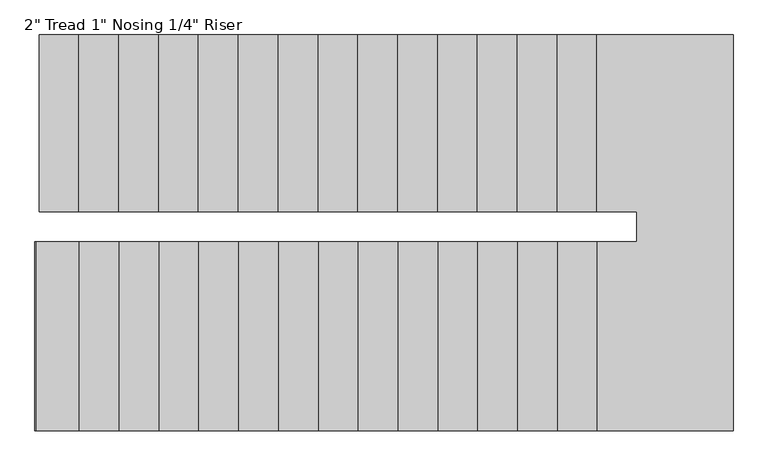
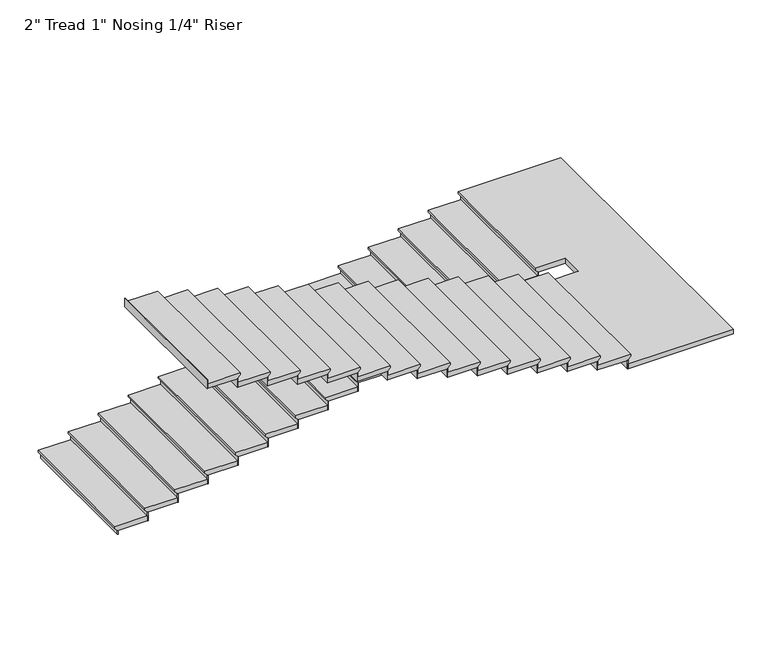
"""IFC4 building model written with IfcOpenShell, lengths in millimetres: stair flight geometry."""

from ifc_helpers import new_model, si_unit, origin, place, context, project, spatial, faceted_brep, source, transform, mapped, element, save


def stair_flight_175a6785(model_context):
    return source(origin(), model_context, "Body", "Brep", [
        faceted_brep([(-5254.0891351, 11154.2082924, 3120.39), (-5254.0891351, 11154.2082924, 3139.44), (-5254.0891351, 12506.0715905, 3139.44), (-5254.0891351, 12506.0715905, 3120.39), (-5228.6891351, 11154.2082924, 3094.99), (-5228.6891351, 12506.0715905, 3094.99), (-4923.8891351, 11154.2082924, 3139.44), (-4923.8891351, 12506.0715905, 3139.44), (-5228.6891351, 12506.0715905, 3088.64), (-4923.8891351, 12506.0715905, 3088.64), (-4923.8891351, 11154.2082924, 3088.64), (-5228.6891351, 11154.2082924, 3088.64)], [[[0, 1, 2, 3]], [[4, 0, 3, 5]], [[2, 1, 6, 7]], [[8, 9, 10, 11]], [[2, 7, 9, 8, 5, 3]], [[8, 11, 4, 5]], [[6, 1, 0, 4, 11, 10]], [[7, 6, 10, 9]]]),
        faceted_brep([(-5228.6891351, 11154.2082924, 3088.64), (-5228.6891351, 11154.2082924, 3048.0), (-5222.3391351, 11154.2082924, 3048.0), (-5222.3391351, 11154.2082924, 3088.64), (-5228.6891351, 12506.0715905, 3088.64), (-5222.3391351, 12506.0715905, 3088.64), (-5222.3391351, 12506.0715905, 3048.0), (-5228.6891351, 12506.0715905, 3048.0)], [[[0, 1, 2, 3]], [[4, 5, 6, 7]], [[1, 0, 4, 7]], [[2, 1, 7, 6]], [[3, 2, 6, 5]], [[0, 3, 5, 4]]]),
        faceted_brep([(-4923.8891351, 11154.2082924, 3180.08), (-4923.8891351, 11154.2082924, 3088.64), (-4917.5391351, 11154.2082924, 3088.64), (-4917.5391351, 11154.2082924, 3180.08), (-4923.8891351, 12506.0715905, 3180.08), (-4917.5391351, 12506.0715905, 3180.08), (-4917.5391351, 12506.0715905, 3088.64), (-4923.8891351, 12506.0715905, 3088.64)], [[[0, 1, 2, 3]], [[4, 5, 6, 7]], [[1, 0, 4, 7]], [[2, 1, 7, 6]], [[3, 2, 6, 5]], [[0, 3, 5, 4]]]),
        faceted_brep([(-4949.2891351, 12506.0715905, 3230.88), (-4949.2891351, 11154.2082924, 3230.88), (-4619.0891351, 11154.2082924, 3230.88), (-4619.0891351, 12506.0715905, 3230.88), (-4923.8891351, 12506.0715905, 3180.08), (-4619.0891351, 12506.0715905, 3180.08), (-4619.0891351, 11154.2082924, 3180.08), (-4923.8891351, 11154.2082924, 3180.08), (-4923.8891351, 12506.0715905, 3186.43), (-4949.2891351, 12506.0715905, 3211.83), (-4923.8891351, 11154.2082924, 3186.43), (-4949.2891351, 11154.2082924, 3211.83)], [[[0, 1, 2, 3]], [[4, 5, 6, 7]], [[0, 3, 5, 4, 8, 9]], [[4, 7, 10, 8]], [[2, 1, 11, 10, 7, 6]], [[3, 2, 6, 5]], [[11, 1, 0, 9]], [[10, 11, 9, 8]]]),
        faceted_brep([(-4619.0891351, 11154.2082924, 3271.52), (-4619.0891351, 11154.2082924, 3180.08), (-4612.7391351, 11154.2082924, 3180.08), (-4612.7391351, 11154.2082924, 3271.52), (-4619.0891351, 12506.0715905, 3271.52), (-4612.7391351, 12506.0715905, 3271.52), (-4612.7391351, 12506.0715905, 3180.08), (-4619.0891351, 12506.0715905, 3180.08)], [[[0, 1, 2, 3]], [[4, 5, 6, 7]], [[1, 0, 4, 7]], [[2, 1, 7, 6]], [[3, 2, 6, 5]], [[0, 3, 5, 4]]]),
        faceted_brep([(-4644.4891351, 12506.0715905, 3322.32), (-4644.4891351, 11154.2082924, 3322.32), (-4314.2891351, 11154.2082924, 3322.32), (-4314.2891351, 12506.0715905, 3322.32), (-4619.0891351, 12506.0715905, 3271.52), (-4314.2891351, 12506.0715905, 3271.52), (-4314.2891351, 11154.2082924, 3271.52), (-4619.0891351, 11154.2082924, 3271.52), (-4619.0891351, 12506.0715905, 3277.87), (-4644.4891351, 12506.0715905, 3303.27), (-4619.0891351, 11154.2082924, 3277.87), (-4644.4891351, 11154.2082924, 3303.27)], [[[0, 1, 2, 3]], [[4, 5, 6, 7]], [[0, 3, 5, 4, 8, 9]], [[4, 7, 10, 8]], [[2, 1, 11, 10, 7, 6]], [[3, 2, 6, 5]], [[11, 1, 0, 9]], [[10, 11, 9, 8]]]),
        faceted_brep([(-4314.2891351, 11154.2082924, 3362.96), (-4314.2891351, 11154.2082924, 3271.52), (-4307.9391351, 11154.2082924, 3271.52), (-4307.9391351, 11154.2082924, 3362.96), (-4314.2891351, 12506.0715905, 3362.96), (-4307.9391351, 12506.0715905, 3362.96), (-4307.9391351, 12506.0715905, 3271.52), (-4314.2891351, 12506.0715905, 3271.52)], [[[0, 1, 2, 3]], [[4, 5, 6, 7]], [[1, 0, 4, 7]], [[2, 1, 7, 6]], [[3, 2, 6, 5]], [[0, 3, 5, 4]]]),
        faceted_brep([(-4339.6891351, 12506.0715905, 3413.76), (-4339.6891351, 11154.2082924, 3413.76), (-4009.4891351, 11154.2082924, 3413.76), (-4009.4891351, 12506.0715905, 3413.76), (-4314.2891351, 12506.0715905, 3362.96), (-4009.4891351, 12506.0715905, 3362.96), (-4009.4891351, 11154.2082924, 3362.96), (-4314.2891351, 11154.2082924, 3362.96), (-4314.2891351, 12506.0715905, 3369.31), (-4339.6891351, 12506.0715905, 3394.71), (-4314.2891351, 11154.2082924, 3369.31), (-4339.6891351, 11154.2082924, 3394.71)], [[[0, 1, 2, 3]], [[4, 5, 6, 7]], [[0, 3, 5, 4, 8, 9]], [[4, 7, 10, 8]], [[2, 1, 11, 10, 7, 6]], [[3, 2, 6, 5]], [[11, 1, 0, 9]], [[10, 11, 9, 8]]]),
        faceted_brep([(-4009.4891351, 11154.2082924, 3454.4), (-4009.4891351, 11154.2082924, 3362.96), (-4003.1391351, 11154.2082924, 3362.96), (-4003.1391351, 11154.2082924, 3454.4), (-4009.4891351, 12506.0715905, 3454.4), (-4003.1391351, 12506.0715905, 3454.4), (-4003.1391351, 12506.0715905, 3362.96), (-4009.4891351, 12506.0715905, 3362.96)], [[[0, 1, 2, 3]], [[4, 5, 6, 7]], [[1, 0, 4, 7]], [[2, 1, 7, 6]], [[3, 2, 6, 5]], [[0, 3, 5, 4]]]),
        faceted_brep([(-4034.8891351, 12506.0715905, 3505.2), (-4034.8891351, 11154.2082924, 3505.2), (-3704.6891351, 11154.2082924, 3505.2), (-3704.6891351, 12506.0715905, 3505.2), (-4009.4891351, 12506.0715905, 3454.4), (-3704.6891351, 12506.0715905, 3454.4), (-3704.6891351, 11154.2082924, 3454.4), (-4009.4891351, 11154.2082924, 3454.4), (-4009.4891351, 12506.0715905, 3460.75), (-4034.8891351, 12506.0715905, 3486.15), (-4009.4891351, 11154.2082924, 3460.75), (-4034.8891351, 11154.2082924, 3486.15)], [[[0, 1, 2, 3]], [[4, 5, 6, 7]], [[0, 3, 5, 4, 8, 9]], [[4, 7, 10, 8]], [[2, 1, 11, 10, 7, 6]], [[3, 2, 6, 5]], [[11, 1, 0, 9]], [[10, 11, 9, 8]]]),
        faceted_brep([(-3704.6891351, 11154.2082924, 3545.84), (-3704.6891351, 11154.2082924, 3454.4), (-3698.3391351, 11154.2082924, 3454.4), (-3698.3391351, 11154.2082924, 3545.84), (-3704.6891351, 12506.0715905, 3545.84), (-3698.3391351, 12506.0715905, 3545.84), (-3698.3391351, 12506.0715905, 3454.4), (-3704.6891351, 12506.0715905, 3454.4)], [[[0, 1, 2, 3]], [[4, 5, 6, 7]], [[1, 0, 4, 7]], [[2, 1, 7, 6]], [[3, 2, 6, 5]], [[0, 3, 5, 4]]]),
        faceted_brep([(-3730.0891351, 12506.0715905, 3596.64), (-3730.0891351, 11154.2082924, 3596.64), (-3399.8891351, 11154.2082924, 3596.64), (-3399.8891351, 12506.0715905, 3596.64), (-3704.6891351, 12506.0715905, 3545.84), (-3399.8891351, 12506.0715905, 3545.84), (-3399.8891351, 11154.2082924, 3545.84), (-3704.6891351, 11154.2082924, 3545.84), (-3704.6891351, 12506.0715905, 3552.19), (-3730.0891351, 12506.0715905, 3577.59), (-3704.6891351, 11154.2082924, 3552.19), (-3730.0891351, 11154.2082924, 3577.59)], [[[0, 1, 2, 3]], [[4, 5, 6, 7]], [[0, 3, 5, 4, 8, 9]], [[4, 7, 10, 8]], [[2, 1, 11, 10, 7, 6]], [[3, 2, 6, 5]], [[11, 1, 0, 9]], [[10, 11, 9, 8]]]),
        faceted_brep([(-3399.8891351, 11154.2082924, 3637.28), (-3399.8891351, 11154.2082924, 3545.84), (-3393.5391351, 11154.2082924, 3545.84), (-3393.5391351, 11154.2082924, 3637.28), (-3399.8891351, 12506.0715905, 3637.28), (-3393.5391351, 12506.0715905, 3637.28), (-3393.5391351, 12506.0715905, 3545.84), (-3399.8891351, 12506.0715905, 3545.84)], [[[0, 1, 2, 3]], [[4, 5, 6, 7]], [[1, 0, 4, 7]], [[2, 1, 7, 6]], [[3, 2, 6, 5]], [[0, 3, 5, 4]]]),
        faceted_brep([(-3425.2891351, 12506.0715905, 3688.08), (-3425.2891351, 11154.2082924, 3688.08), (-3095.0891351, 11154.2082924, 3688.08), (-3095.0891351, 12506.0715905, 3688.08), (-3399.8891351, 12506.0715905, 3637.28), (-3095.0891351, 12506.0715905, 3637.28), (-3095.0891351, 11154.2082924, 3637.28), (-3399.8891351, 11154.2082924, 3637.28), (-3399.8891351, 12506.0715905, 3643.63), (-3425.2891351, 12506.0715905, 3669.03), (-3399.8891351, 11154.2082924, 3643.63), (-3425.2891351, 11154.2082924, 3669.03)], [[[0, 1, 2, 3]], [[4, 5, 6, 7]], [[0, 3, 5, 4, 8, 9]], [[4, 7, 10, 8]], [[2, 1, 11, 10, 7, 6]], [[3, 2, 6, 5]], [[11, 1, 0, 9]], [[10, 11, 9, 8]]]),
        faceted_brep([(-3095.0891351, 11154.2082924, 3728.72), (-3095.0891351, 11154.2082924, 3637.28), (-3088.7391351, 11154.2082924, 3637.28), (-3088.7391351, 11154.2082924, 3728.72), (-3095.0891351, 12506.0715905, 3728.72), (-3088.7391351, 12506.0715905, 3728.72), (-3088.7391351, 12506.0715905, 3637.28), (-3095.0891351, 12506.0715905, 3637.28)], [[[0, 1, 2, 3]], [[4, 5, 6, 7]], [[1, 0, 4, 7]], [[2, 1, 7, 6]], [[3, 2, 6, 5]], [[0, 3, 5, 4]]]),
        faceted_brep([(-3120.4891351, 12506.0715905, 3779.52), (-3120.4891351, 11154.2082924, 3779.52), (-2790.2891351, 11154.2082924, 3779.52), (-2790.2891351, 12506.0715905, 3779.52), (-3095.0891351, 12506.0715905, 3728.72), (-2790.2891351, 12506.0715905, 3728.72), (-2790.2891351, 11154.2082924, 3728.72), (-3095.0891351, 11154.2082924, 3728.72), (-3095.0891351, 12506.0715905, 3735.07), (-3120.4891351, 12506.0715905, 3760.47), (-3095.0891351, 11154.2082924, 3735.07), (-3120.4891351, 11154.2082924, 3760.47)], [[[0, 1, 2, 3]], [[4, 5, 6, 7]], [[0, 3, 5, 4, 8, 9]], [[4, 7, 10, 8]], [[2, 1, 11, 10, 7, 6]], [[3, 2, 6, 5]], [[11, 1, 0, 9]], [[10, 11, 9, 8]]]),
        faceted_brep([(-2790.2891351, 11154.2082924, 3820.16), (-2790.2891351, 11154.2082924, 3728.72), (-2783.9391351, 11154.2082924, 3728.72), (-2783.9391351, 11154.2082924, 3820.16), (-2790.2891351, 12506.0715905, 3820.16), (-2783.9391351, 12506.0715905, 3820.16), (-2783.9391351, 12506.0715905, 3728.72), (-2790.2891351, 12506.0715905, 3728.72)], [[[0, 1, 2, 3]], [[4, 5, 6, 7]], [[1, 0, 4, 7]], [[2, 1, 7, 6]], [[3, 2, 6, 5]], [[0, 3, 5, 4]]]),
        faceted_brep([(-2815.6891351, 12506.0715905, 3870.96), (-2815.6891351, 11154.2082924, 3870.96), (-2485.4891351, 11154.2082924, 3870.96), (-2485.4891351, 12506.0715905, 3870.96), (-2790.2891351, 12506.0715905, 3820.16), (-2485.4891351, 12506.0715905, 3820.16), (-2485.4891351, 11154.2082924, 3820.16), (-2790.2891351, 11154.2082924, 3820.16), (-2790.2891351, 12506.0715905, 3826.51), (-2815.6891351, 12506.0715905, 3851.91), (-2790.2891351, 11154.2082924, 3826.51), (-2815.6891351, 11154.2082924, 3851.91)], [[[0, 1, 2, 3]], [[4, 5, 6, 7]], [[0, 3, 5, 4, 8, 9]], [[4, 7, 10, 8]], [[2, 1, 11, 10, 7, 6]], [[3, 2, 6, 5]], [[11, 1, 0, 9]], [[10, 11, 9, 8]]]),
        faceted_brep([(-2485.4891351, 11154.2082924, 3911.6), (-2485.4891351, 11154.2082924, 3820.16), (-2479.1391351, 11154.2082924, 3820.16), (-2479.1391351, 11154.2082924, 3911.6), (-2485.4891351, 12506.0715905, 3911.6), (-2479.1391351, 12506.0715905, 3911.6), (-2479.1391351, 12506.0715905, 3820.16), (-2485.4891351, 12506.0715905, 3820.16)], [[[0, 1, 2, 3]], [[4, 5, 6, 7]], [[1, 0, 4, 7]], [[2, 1, 7, 6]], [[3, 2, 6, 5]], [[0, 3, 5, 4]]]),
        faceted_brep([(-2510.8891351, 12506.0715905, 3962.4), (-2510.8891351, 11154.2082924, 3962.4), (-2180.6891351, 11154.2082924, 3962.4), (-2180.6891351, 12506.0715905, 3962.4), (-2485.4891351, 12506.0715905, 3911.6), (-2180.6891351, 12506.0715905, 3911.6), (-2180.6891351, 11154.2082924, 3911.6), (-2485.4891351, 11154.2082924, 3911.6), (-2485.4891351, 12506.0715905, 3917.95), (-2510.8891351, 12506.0715905, 3943.35), (-2485.4891351, 11154.2082924, 3917.95), (-2510.8891351, 11154.2082924, 3943.35)], [[[0, 1, 2, 3]], [[4, 5, 6, 7]], [[0, 3, 5, 4, 8, 9]], [[4, 7, 10, 8]], [[2, 1, 11, 10, 7, 6]], [[3, 2, 6, 5]], [[11, 1, 0, 9]], [[10, 11, 9, 8]]]),
        faceted_brep([(-2180.6891351, 11154.2082924, 4003.04), (-2180.6891351, 11154.2082924, 3911.6), (-2174.3391351, 11154.2082924, 3911.6), (-2174.3391351, 11154.2082924, 4003.04), (-2180.6891351, 12506.0715905, 4003.04), (-2174.3391351, 12506.0715905, 4003.04), (-2174.3391351, 12506.0715905, 3911.6), (-2180.6891351, 12506.0715905, 3911.6)], [[[0, 1, 2, 3]], [[4, 5, 6, 7]], [[1, 0, 4, 7]], [[2, 1, 7, 6]], [[3, 2, 6, 5]], [[0, 3, 5, 4]]]),
        faceted_brep([(-2206.0891351, 12506.0715905, 4053.84), (-2206.0891351, 11154.2082924, 4053.84), (-1875.8891351, 11154.2082924, 4053.84), (-1875.8891351, 12506.0715905, 4053.84), (-2180.6891351, 12506.0715905, 4003.04), (-1875.8891351, 12506.0715905, 4003.04), (-1875.8891351, 11154.2082924, 4003.04), (-2180.6891351, 11154.2082924, 4003.04), (-2180.6891351, 12506.0715905, 4009.39), (-2206.0891351, 12506.0715905, 4034.79), (-2180.6891351, 11154.2082924, 4009.39), (-2206.0891351, 11154.2082924, 4034.79)], [[[0, 1, 2, 3]], [[4, 5, 6, 7]], [[0, 3, 5, 4, 8, 9]], [[4, 7, 10, 8]], [[2, 1, 11, 10, 7, 6]], [[3, 2, 6, 5]], [[11, 1, 0, 9]], [[10, 11, 9, 8]]]),
        faceted_brep([(-1875.8891351, 11154.2082924, 4094.48), (-1875.8891351, 11154.2082924, 4003.04), (-1869.5391351, 11154.2082924, 4003.04), (-1869.5391351, 11154.2082924, 4094.48), (-1875.8891351, 12506.0715905, 4094.48), (-1869.5391351, 12506.0715905, 4094.48), (-1869.5391351, 12506.0715905, 4003.04), (-1875.8891351, 12506.0715905, 4003.04)], [[[0, 1, 2, 3]], [[4, 5, 6, 7]], [[1, 0, 4, 7]], [[2, 1, 7, 6]], [[3, 2, 6, 5]], [[0, 3, 5, 4]]]),
        faceted_brep([(-1901.2891351, 12506.0715905, 4145.28), (-1901.2891351, 11154.2082924, 4145.28), (-1571.0891351, 11154.2082924, 4145.28), (-1571.0891351, 12506.0715905, 4145.28), (-1875.8891351, 12506.0715905, 4094.48), (-1571.0891351, 12506.0715905, 4094.48), (-1571.0891351, 11154.2082924, 4094.48), (-1875.8891351, 11154.2082924, 4094.48), (-1875.8891351, 12506.0715905, 4100.83), (-1901.2891351, 12506.0715905, 4126.23), (-1875.8891351, 11154.2082924, 4100.83), (-1901.2891351, 11154.2082924, 4126.23)], [[[0, 1, 2, 3]], [[4, 5, 6, 7]], [[0, 3, 5, 4, 8, 9]], [[4, 7, 10, 8]], [[2, 1, 11, 10, 7, 6]], [[3, 2, 6, 5]], [[11, 1, 0, 9]], [[10, 11, 9, 8]]]),
        faceted_brep([(-1571.0891351, 11154.2082924, 4185.92), (-1571.0891351, 11154.2082924, 4094.48), (-1564.7391351, 11154.2082924, 4094.48), (-1564.7391351, 11154.2082924, 4185.92), (-1571.0891351, 12506.0715905, 4185.92), (-1564.7391351, 12506.0715905, 4185.92), (-1564.7391351, 12506.0715905, 4094.48), (-1571.0891351, 12506.0715905, 4094.48)], [[[0, 1, 2, 3]], [[4, 5, 6, 7]], [[1, 0, 4, 7]], [[2, 1, 7, 6]], [[3, 2, 6, 5]], [[0, 3, 5, 4]]]),
        faceted_brep([(-1596.4891351, 12506.0715905, 4236.72), (-1596.4891351, 11154.2082924, 4236.72), (-1266.2891351, 11154.2082924, 4236.72), (-1266.2891351, 12506.0715905, 4236.72), (-1571.0891351, 12506.0715905, 4185.92), (-1266.2891351, 12506.0715905, 4185.92), (-1266.2891351, 11154.2082924, 4185.92), (-1571.0891351, 11154.2082924, 4185.92), (-1571.0891351, 12506.0715905, 4192.27), (-1596.4891351, 12506.0715905, 4217.67), (-1571.0891351, 11154.2082924, 4192.27), (-1596.4891351, 11154.2082924, 4217.67)], [[[0, 1, 2, 3]], [[4, 5, 6, 7]], [[0, 3, 5, 4, 8, 9]], [[4, 7, 10, 8]], [[2, 1, 11, 10, 7, 6]], [[3, 2, 6, 5]], [[11, 1, 0, 9]], [[10, 11, 9, 8]]]),
        faceted_brep([(-1266.2891351, 11154.2082924, 4277.36), (-1266.2891351, 11154.2082924, 4185.92), (-1259.9391351, 11154.2082924, 4185.92), (-1259.9391351, 11154.2082924, 4277.36), (-1266.2891351, 12506.0715905, 4277.36), (-1259.9391351, 12506.0715905, 4277.36), (-1259.9391351, 12506.0715905, 4185.92), (-1266.2891351, 12506.0715905, 4185.92)], [[[0, 1, 2, 3]], [[4, 5, 6, 7]], [[1, 0, 4, 7]], [[2, 1, 7, 6]], [[3, 2, 6, 5]], [[0, 3, 5, 4]]]),
        faceted_brep([(-1291.6891351, 12506.0715905, 4328.16), (-1291.6891351, 11154.2082924, 4328.16), (-961.4891351, 11154.2082924, 4328.16), (-961.4891351, 12506.0715905, 4328.16), (-1266.2891351, 12506.0715905, 4277.36), (-961.4891351, 12506.0715905, 4277.36), (-961.4891351, 11154.2082924, 4277.36), (-1266.2891351, 11154.2082924, 4277.36), (-1266.2891351, 12506.0715905, 4283.71), (-1291.6891351, 12506.0715905, 4309.11), (-1266.2891351, 11154.2082924, 4283.71), (-1291.6891351, 11154.2082924, 4309.11)], [[[0, 1, 2, 3]], [[4, 5, 6, 7]], [[0, 3, 5, 4, 8, 9]], [[4, 7, 10, 8]], [[2, 1, 11, 10, 7, 6]], [[3, 2, 6, 5]], [[11, 1, 0, 9]], [[10, 11, 9, 8]]]),
        faceted_brep([(-961.4891351, 11154.2082924, 4368.8), (-961.4891351, 11154.2082924, 4277.36), (-955.1391351, 11154.2082924, 4277.36), (-955.1391351, 11154.2082924, 4368.8), (-961.4891351, 12506.0715905, 4368.8), (-955.1391351, 12506.0715905, 4368.8), (-955.1391351, 12506.0715905, 4277.36), (-961.4891351, 12506.0715905, 4277.36)], [[[0, 1, 2, 3]], [[4, 5, 6, 7]], [[1, 0, 4, 7]], [[2, 1, 7, 6]], [[3, 2, 6, 5]], [[0, 3, 5, 4]]]),
        faceted_brep([(-1012.2891351, 9478.4949943, 4419.6), (54.5108649, 9478.4949943, 4419.6), (54.5108649, 12506.0715905, 4419.6), (-986.8891351, 12506.0715905, 4419.6), (-986.8891351, 11154.2082924, 4419.6), (-682.0891351, 11154.2082924, 4419.6), (-682.0891351, 10925.6082924, 4419.6), (-1012.2891351, 10925.6082924, 4419.6), (54.5108649, 9478.4949943, 4368.8), (-1012.2891351, 9478.4949943, 4368.8), (-1012.2891351, 10925.6082924, 4368.8), (-682.0891351, 10925.6082924, 4368.8), (-682.0891351, 11154.2082924, 4368.8), (-961.4891351, 11154.2082924, 4368.8), (-961.4891351, 12506.0715905, 4368.8), (54.5108649, 12506.0715905, 4368.8), (-961.4891351, 12506.0715905, 4375.15), (-986.8891351, 12506.0715905, 4400.55), (-961.4891351, 11154.2082924, 4375.15), (-986.8891351, 11154.2082924, 4400.55)], [[[0, 1, 2, 3, 4, 5, 6, 7]], [[8, 9, 10, 11, 12, 13, 14, 15]], [[1, 0, 9, 8]], [[2, 1, 8, 15]], [[3, 2, 15, 14, 16, 17]], [[14, 13, 18, 16]], [[5, 4, 19, 18, 13, 12]], [[6, 5, 12, 11]], [[7, 6, 11, 10]], [[0, 7, 10, 9]], [[19, 4, 3, 17]], [[18, 19, 17, 16]]]),
        faceted_brep([(-1012.2891351, 10925.6082924, 4460.24), (-1012.2891351, 10925.6082924, 4368.8), (-1018.6391351, 10925.6082924, 4368.8), (-1018.6391351, 10925.6082924, 4460.24), (-1012.2891351, 9478.4949943, 4460.24), (-1018.6391351, 9478.4949943, 4460.24), (-1018.6391351, 9478.4949943, 4368.8), (-1012.2891351, 9478.4949943, 4368.8)], [[[0, 1, 2, 3]], [[4, 5, 6, 7]], [[1, 0, 4, 7]], [[2, 1, 7, 6]], [[3, 2, 6, 5]], [[0, 3, 5, 4]]]),
        faceted_brep([(-986.8891351, 9478.4949943, 4511.04), (-986.8891351, 10925.6082924, 4511.04), (-1317.0891351, 10925.6082924, 4511.04), (-1317.0891351, 9478.4949943, 4511.04), (-1012.2891351, 9478.4949943, 4460.24), (-1317.0891351, 9478.4949943, 4460.24), (-1317.0891351, 10925.6082924, 4460.24), (-1012.2891351, 10925.6082924, 4460.24), (-1012.2891351, 9478.4949943, 4466.59), (-986.8891351, 9478.4949943, 4491.99), (-1012.2891351, 10925.6082924, 4466.59), (-986.8891351, 10925.6082924, 4491.99)], [[[0, 1, 2, 3]], [[4, 5, 6, 7]], [[0, 3, 5, 4, 8, 9]], [[4, 7, 10, 8]], [[2, 1, 11, 10, 7, 6]], [[3, 2, 6, 5]], [[11, 1, 0, 9]], [[10, 11, 9, 8]]]),
        faceted_brep([(-1317.0891351, 10925.6082924, 4551.68), (-1317.0891351, 10925.6082924, 4460.24), (-1323.4391351, 10925.6082924, 4460.24), (-1323.4391351, 10925.6082924, 4551.68), (-1317.0891351, 9478.4949943, 4551.68), (-1323.4391351, 9478.4949943, 4551.68), (-1323.4391351, 9478.4949943, 4460.24), (-1317.0891351, 9478.4949943, 4460.24)], [[[0, 1, 2, 3]], [[4, 5, 6, 7]], [[1, 0, 4, 7]], [[2, 1, 7, 6]], [[3, 2, 6, 5]], [[0, 3, 5, 4]]]),
        faceted_brep([(-1291.6891351, 9478.4949943, 4602.48), (-1291.6891351, 10925.6082924, 4602.48), (-1621.8891351, 10925.6082924, 4602.48), (-1621.8891351, 9478.4949943, 4602.48), (-1317.0891351, 9478.4949943, 4551.68), (-1621.8891351, 9478.4949943, 4551.68), (-1621.8891351, 10925.6082924, 4551.68), (-1317.0891351, 10925.6082924, 4551.68), (-1317.0891351, 9478.4949943, 4558.03), (-1291.6891351, 9478.4949943, 4583.43), (-1317.0891351, 10925.6082924, 4558.03), (-1291.6891351, 10925.6082924, 4583.43)], [[[0, 1, 2, 3]], [[4, 5, 6, 7]], [[0, 3, 5, 4, 8, 9]], [[4, 7, 10, 8]], [[2, 1, 11, 10, 7, 6]], [[3, 2, 6, 5]], [[11, 1, 0, 9]], [[10, 11, 9, 8]]]),
        faceted_brep([(-1621.8891351, 10925.6082924, 4643.12), (-1621.8891351, 10925.6082924, 4551.68), (-1628.2391351, 10925.6082924, 4551.68), (-1628.2391351, 10925.6082924, 4643.12), (-1621.8891351, 9478.4949943, 4643.12), (-1628.2391351, 9478.4949943, 4643.12), (-1628.2391351, 9478.4949943, 4551.68), (-1621.8891351, 9478.4949943, 4551.68)], [[[0, 1, 2, 3]], [[4, 5, 6, 7]], [[1, 0, 4, 7]], [[2, 1, 7, 6]], [[3, 2, 6, 5]], [[0, 3, 5, 4]]]),
        faceted_brep([(-1596.4891351, 9478.4949943, 4693.92), (-1596.4891351, 10925.6082924, 4693.92), (-1926.6891351, 10925.6082924, 4693.92), (-1926.6891351, 9478.4949943, 4693.92), (-1621.8891351, 9478.4949943, 4643.12), (-1926.6891351, 9478.4949943, 4643.12), (-1926.6891351, 10925.6082924, 4643.12), (-1621.8891351, 10925.6082924, 4643.12), (-1621.8891351, 9478.4949943, 4649.47), (-1596.4891351, 9478.4949943, 4674.87), (-1621.8891351, 10925.6082924, 4649.47), (-1596.4891351, 10925.6082924, 4674.87)], [[[0, 1, 2, 3]], [[4, 5, 6, 7]], [[0, 3, 5, 4, 8, 9]], [[4, 7, 10, 8]], [[2, 1, 11, 10, 7, 6]], [[3, 2, 6, 5]], [[11, 1, 0, 9]], [[10, 11, 9, 8]]]),
        faceted_brep([(-1926.6891351, 10925.6082924, 4734.56), (-1926.6891351, 10925.6082924, 4643.12), (-1933.0391351, 10925.6082924, 4643.12), (-1933.0391351, 10925.6082924, 4734.56), (-1926.6891351, 9478.4949943, 4734.56), (-1933.0391351, 9478.4949943, 4734.56), (-1933.0391351, 9478.4949943, 4643.12), (-1926.6891351, 9478.4949943, 4643.12)], [[[0, 1, 2, 3]], [[4, 5, 6, 7]], [[1, 0, 4, 7]], [[2, 1, 7, 6]], [[3, 2, 6, 5]], [[0, 3, 5, 4]]]),
        faceted_brep([(-1901.2891351, 9478.4949943, 4785.36), (-1901.2891351, 10925.6082924, 4785.36), (-2231.4891351, 10925.6082924, 4785.36), (-2231.4891351, 9478.4949943, 4785.36), (-1926.6891351, 9478.4949943, 4734.56), (-2231.4891351, 9478.4949943, 4734.56), (-2231.4891351, 10925.6082924, 4734.56), (-1926.6891351, 10925.6082924, 4734.56), (-1926.6891351, 9478.4949943, 4740.91), (-1901.2891351, 9478.4949943, 4766.31), (-1926.6891351, 10925.6082924, 4740.91), (-1901.2891351, 10925.6082924, 4766.31)], [[[0, 1, 2, 3]], [[4, 5, 6, 7]], [[0, 3, 5, 4, 8, 9]], [[4, 7, 10, 8]], [[2, 1, 11, 10, 7, 6]], [[3, 2, 6, 5]], [[11, 1, 0, 9]], [[10, 11, 9, 8]]]),
        faceted_brep([(-2231.4891351, 10925.6082924, 4826.0), (-2231.4891351, 10925.6082924, 4734.56), (-2237.8391351, 10925.6082924, 4734.56), (-2237.8391351, 10925.6082924, 4826.0), (-2231.4891351, 9478.4949943, 4826.0), (-2237.8391351, 9478.4949943, 4826.0), (-2237.8391351, 9478.4949943, 4734.56), (-2231.4891351, 9478.4949943, 4734.56)], [[[0, 1, 2, 3]], [[4, 5, 6, 7]], [[1, 0, 4, 7]], [[2, 1, 7, 6]], [[3, 2, 6, 5]], [[0, 3, 5, 4]]]),
        faceted_brep([(-2206.0891351, 9478.4949943, 4876.8), (-2206.0891351, 10925.6082924, 4876.8), (-2536.2891351, 10925.6082924, 4876.8), (-2536.2891351, 9478.4949943, 4876.8), (-2231.4891351, 9478.4949943, 4826.0), (-2536.2891351, 9478.4949943, 4826.0), (-2536.2891351, 10925.6082924, 4826.0), (-2231.4891351, 10925.6082924, 4826.0), (-2231.4891351, 9478.4949943, 4832.35), (-2206.0891351, 9478.4949943, 4857.75), (-2231.4891351, 10925.6082924, 4832.35), (-2206.0891351, 10925.6082924, 4857.75)], [[[0, 1, 2, 3]], [[4, 5, 6, 7]], [[0, 3, 5, 4, 8, 9]], [[4, 7, 10, 8]], [[2, 1, 11, 10, 7, 6]], [[3, 2, 6, 5]], [[11, 1, 0, 9]], [[10, 11, 9, 8]]]),
        faceted_brep([(-2536.2891351, 10925.6082924, 4917.44), (-2536.2891351, 10925.6082924, 4826.0), (-2542.6391351, 10925.6082924, 4826.0), (-2542.6391351, 10925.6082924, 4917.44), (-2536.2891351, 9478.4949943, 4917.44), (-2542.6391351, 9478.4949943, 4917.44), (-2542.6391351, 9478.4949943, 4826.0), (-2536.2891351, 9478.4949943, 4826.0)], [[[0, 1, 2, 3]], [[4, 5, 6, 7]], [[1, 0, 4, 7]], [[2, 1, 7, 6]], [[3, 2, 6, 5]], [[0, 3, 5, 4]]]),
        faceted_brep([(-2510.8891351, 9478.4949943, 4968.24), (-2510.8891351, 10925.6082924, 4968.24), (-2841.0891351, 10925.6082924, 4968.24), (-2841.0891351, 9478.4949943, 4968.24), (-2536.2891351, 9478.4949943, 4917.44), (-2841.0891351, 9478.4949943, 4917.44), (-2841.0891351, 10925.6082924, 4917.44), (-2536.2891351, 10925.6082924, 4917.44), (-2536.2891351, 9478.4949943, 4923.79), (-2510.8891351, 9478.4949943, 4949.19), (-2536.2891351, 10925.6082924, 4923.79), (-2510.8891351, 10925.6082924, 4949.19)], [[[0, 1, 2, 3]], [[4, 5, 6, 7]], [[0, 3, 5, 4, 8, 9]], [[4, 7, 10, 8]], [[2, 1, 11, 10, 7, 6]], [[3, 2, 6, 5]], [[11, 1, 0, 9]], [[10, 11, 9, 8]]]),
        faceted_brep([(-2841.0891351, 10925.6082924, 5008.88), (-2841.0891351, 10925.6082924, 4917.44), (-2847.4391351, 10925.6082924, 4917.44), (-2847.4391351, 10925.6082924, 5008.88), (-2841.0891351, 9478.4949943, 5008.88), (-2847.4391351, 9478.4949943, 5008.88), (-2847.4391351, 9478.4949943, 4917.44), (-2841.0891351, 9478.4949943, 4917.44)], [[[0, 1, 2, 3]], [[4, 5, 6, 7]], [[1, 0, 4, 7]], [[2, 1, 7, 6]], [[3, 2, 6, 5]], [[0, 3, 5, 4]]]),
        faceted_brep([(-2815.6891351, 9478.4949943, 5059.68), (-2815.6891351, 10925.6082924, 5059.68), (-3145.8891351, 10925.6082924, 5059.68), (-3145.8891351, 9478.4949943, 5059.68), (-2841.0891351, 9478.4949943, 5008.88), (-3145.8891351, 9478.4949943, 5008.88), (-3145.8891351, 10925.6082924, 5008.88), (-2841.0891351, 10925.6082924, 5008.88), (-2841.0891351, 9478.4949943, 5015.23), (-2815.6891351, 9478.4949943, 5040.63), (-2841.0891351, 10925.6082924, 5015.23), (-2815.6891351, 10925.6082924, 5040.63)], [[[0, 1, 2, 3]], [[4, 5, 6, 7]], [[0, 3, 5, 4, 8, 9]], [[4, 7, 10, 8]], [[2, 1, 11, 10, 7, 6]], [[3, 2, 6, 5]], [[11, 1, 0, 9]], [[10, 11, 9, 8]]]),
        faceted_brep([(-3145.8891351, 10925.6082924, 5100.32), (-3145.8891351, 10925.6082924, 5008.88), (-3152.2391351, 10925.6082924, 5008.88), (-3152.2391351, 10925.6082924, 5100.32), (-3145.8891351, 9478.4949943, 5100.32), (-3152.2391351, 9478.4949943, 5100.32), (-3152.2391351, 9478.4949943, 5008.88), (-3145.8891351, 9478.4949943, 5008.88)], [[[0, 1, 2, 3]], [[4, 5, 6, 7]], [[1, 0, 4, 7]], [[2, 1, 7, 6]], [[3, 2, 6, 5]], [[0, 3, 5, 4]]]),
        faceted_brep([(-3120.4891351, 9478.4949943, 5151.12), (-3120.4891351, 10925.6082924, 5151.12), (-3450.6891351, 10925.6082924, 5151.12), (-3450.6891351, 9478.4949943, 5151.12), (-3145.8891351, 9478.4949943, 5100.32), (-3450.6891351, 9478.4949943, 5100.32), (-3450.6891351, 10925.6082924, 5100.32), (-3145.8891351, 10925.6082924, 5100.32), (-3145.8891351, 9478.4949943, 5106.67), (-3120.4891351, 9478.4949943, 5132.07), (-3145.8891351, 10925.6082924, 5106.67), (-3120.4891351, 10925.6082924, 5132.07)], [[[0, 1, 2, 3]], [[4, 5, 6, 7]], [[0, 3, 5, 4, 8, 9]], [[4, 7, 10, 8]], [[2, 1, 11, 10, 7, 6]], [[3, 2, 6, 5]], [[11, 1, 0, 9]], [[10, 11, 9, 8]]]),
        faceted_brep([(-3450.6891351, 10925.6082924, 5191.76), (-3450.6891351, 10925.6082924, 5100.32), (-3457.0391351, 10925.6082924, 5100.32), (-3457.0391351, 10925.6082924, 5191.76), (-3450.6891351, 9478.4949943, 5191.76), (-3457.0391351, 9478.4949943, 5191.76), (-3457.0391351, 9478.4949943, 5100.32), (-3450.6891351, 9478.4949943, 5100.32)], [[[0, 1, 2, 3]], [[4, 5, 6, 7]], [[1, 0, 4, 7]], [[2, 1, 7, 6]], [[3, 2, 6, 5]], [[0, 3, 5, 4]]]),
        faceted_brep([(-3425.2891351, 9478.4949943, 5242.56), (-3425.2891351, 10925.6082924, 5242.56), (-3755.4891351, 10925.6082924, 5242.56), (-3755.4891351, 9478.4949943, 5242.56), (-3450.6891351, 9478.4949943, 5191.76), (-3755.4891351, 9478.4949943, 5191.76), (-3755.4891351, 10925.6082924, 5191.76), (-3450.6891351, 10925.6082924, 5191.76), (-3450.6891351, 9478.4949943, 5198.11), (-3425.2891351, 9478.4949943, 5223.51), (-3450.6891351, 10925.6082924, 5198.11), (-3425.2891351, 10925.6082924, 5223.51)], [[[0, 1, 2, 3]], [[4, 5, 6, 7]], [[0, 3, 5, 4, 8, 9]], [[4, 7, 10, 8]], [[2, 1, 11, 10, 7, 6]], [[3, 2, 6, 5]], [[11, 1, 0, 9]], [[10, 11, 9, 8]]]),
        faceted_brep([(-3755.4891351, 10925.6082924, 5283.2), (-3755.4891351, 10925.6082924, 5191.76), (-3761.8391351, 10925.6082924, 5191.76), (-3761.8391351, 10925.6082924, 5283.2), (-3755.4891351, 9478.4949943, 5283.2), (-3761.8391351, 9478.4949943, 5283.2), (-3761.8391351, 9478.4949943, 5191.76), (-3755.4891351, 9478.4949943, 5191.76)], [[[0, 1, 2, 3]], [[4, 5, 6, 7]], [[1, 0, 4, 7]], [[2, 1, 7, 6]], [[3, 2, 6, 5]], [[0, 3, 5, 4]]]),
        faceted_brep([(-3730.0891351, 9478.4949943, 5334.0), (-3730.0891351, 10925.6082924, 5334.0), (-4060.2891351, 10925.6082924, 5334.0), (-4060.2891351, 9478.4949943, 5334.0), (-3755.4891351, 9478.4949943, 5283.2), (-4060.2891351, 9478.4949943, 5283.2), (-4060.2891351, 10925.6082924, 5283.2), (-3755.4891351, 10925.6082924, 5283.2), (-3755.4891351, 9478.4949943, 5289.55), (-3730.0891351, 9478.4949943, 5314.95), (-3755.4891351, 10925.6082924, 5289.55), (-3730.0891351, 10925.6082924, 5314.95)], [[[0, 1, 2, 3]], [[4, 5, 6, 7]], [[0, 3, 5, 4, 8, 9]], [[4, 7, 10, 8]], [[2, 1, 11, 10, 7, 6]], [[3, 2, 6, 5]], [[11, 1, 0, 9]], [[10, 11, 9, 8]]]),
        faceted_brep([(-4060.2891351, 10925.6082924, 5374.64), (-4060.2891351, 10925.6082924, 5283.2), (-4066.6391351, 10925.6082924, 5283.2), (-4066.6391351, 10925.6082924, 5374.64), (-4060.2891351, 9478.4949943, 5374.64), (-4066.6391351, 9478.4949943, 5374.64), (-4066.6391351, 9478.4949943, 5283.2), (-4060.2891351, 9478.4949943, 5283.2)], [[[0, 1, 2, 3]], [[4, 5, 6, 7]], [[1, 0, 4, 7]], [[2, 1, 7, 6]], [[3, 2, 6, 5]], [[0, 3, 5, 4]]]),
        faceted_brep([(-4034.8891351, 9478.4949943, 5425.44), (-4034.8891351, 10925.6082924, 5425.44), (-4365.0891351, 10925.6082924, 5425.44), (-4365.0891351, 9478.4949943, 5425.44), (-4060.2891351, 9478.4949943, 5374.64), (-4365.0891351, 9478.4949943, 5374.64), (-4365.0891351, 10925.6082924, 5374.64), (-4060.2891351, 10925.6082924, 5374.64), (-4060.2891351, 9478.4949943, 5380.99), (-4034.8891351, 9478.4949943, 5406.39), (-4060.2891351, 10925.6082924, 5380.99), (-4034.8891351, 10925.6082924, 5406.39)], [[[0, 1, 2, 3]], [[4, 5, 6, 7]], [[0, 3, 5, 4, 8, 9]], [[4, 7, 10, 8]], [[2, 1, 11, 10, 7, 6]], [[3, 2, 6, 5]], [[11, 1, 0, 9]], [[10, 11, 9, 8]]]),
        faceted_brep([(-4365.0891351, 10925.6082924, 5466.08), (-4365.0891351, 10925.6082924, 5374.64), (-4371.4391351, 10925.6082924, 5374.64), (-4371.4391351, 10925.6082924, 5466.08), (-4365.0891351, 9478.4949943, 5466.08), (-4371.4391351, 9478.4949943, 5466.08), (-4371.4391351, 9478.4949943, 5374.64), (-4365.0891351, 9478.4949943, 5374.64)], [[[0, 1, 2, 3]], [[4, 5, 6, 7]], [[1, 0, 4, 7]], [[2, 1, 7, 6]], [[3, 2, 6, 5]], [[0, 3, 5, 4]]]),
        faceted_brep([(-4339.6891351, 9478.4949943, 5516.88), (-4339.6891351, 10925.6082924, 5516.88), (-4669.8891351, 10925.6082924, 5516.88), (-4669.8891351, 9478.4949943, 5516.88), (-4365.0891351, 9478.4949943, 5466.08), (-4669.8891351, 9478.4949943, 5466.08), (-4669.8891351, 10925.6082924, 5466.08), (-4365.0891351, 10925.6082924, 5466.08), (-4365.0891351, 9478.4949943, 5472.43), (-4339.6891351, 9478.4949943, 5497.83), (-4365.0891351, 10925.6082924, 5472.43), (-4339.6891351, 10925.6082924, 5497.83)], [[[0, 1, 2, 3]], [[4, 5, 6, 7]], [[0, 3, 5, 4, 8, 9]], [[4, 7, 10, 8]], [[2, 1, 11, 10, 7, 6]], [[3, 2, 6, 5]], [[11, 1, 0, 9]], [[10, 11, 9, 8]]]),
        faceted_brep([(-4669.8891351, 10925.6082924, 5557.52), (-4669.8891351, 10925.6082924, 5466.08), (-4676.2391351, 10925.6082924, 5466.08), (-4676.2391351, 10925.6082924, 5557.52), (-4669.8891351, 9478.4949943, 5557.52), (-4676.2391351, 9478.4949943, 5557.52), (-4676.2391351, 9478.4949943, 5466.08), (-4669.8891351, 9478.4949943, 5466.08)], [[[0, 1, 2, 3]], [[4, 5, 6, 7]], [[1, 0, 4, 7]], [[2, 1, 7, 6]], [[3, 2, 6, 5]], [[0, 3, 5, 4]]]),
        faceted_brep([(-4644.4891351, 9478.4949943, 5608.32), (-4644.4891351, 10925.6082924, 5608.32), (-4974.6891351, 10925.6082924, 5608.32), (-4974.6891351, 9478.4949943, 5608.32), (-4669.8891351, 9478.4949943, 5557.52), (-4974.6891351, 9478.4949943, 5557.52), (-4974.6891351, 10925.6082924, 5557.52), (-4669.8891351, 10925.6082924, 5557.52), (-4669.8891351, 9478.4949943, 5563.87), (-4644.4891351, 9478.4949943, 5589.27), (-4669.8891351, 10925.6082924, 5563.87), (-4644.4891351, 10925.6082924, 5589.27)], [[[0, 1, 2, 3]], [[4, 5, 6, 7]], [[0, 3, 5, 4, 8, 9]], [[4, 7, 10, 8]], [[2, 1, 11, 10, 7, 6]], [[3, 2, 6, 5]], [[11, 1, 0, 9]], [[10, 11, 9, 8]]]),
        faceted_brep([(-4974.6891351, 10925.6082924, 5648.96), (-4974.6891351, 10925.6082924, 5557.52), (-4981.0391351, 10925.6082924, 5557.52), (-4981.0391351, 10925.6082924, 5648.96), (-4974.6891351, 9478.4949943, 5648.96), (-4981.0391351, 9478.4949943, 5648.96), (-4981.0391351, 9478.4949943, 5557.52), (-4974.6891351, 9478.4949943, 5557.52)], [[[0, 1, 2, 3]], [[4, 5, 6, 7]], [[1, 0, 4, 7]], [[2, 1, 7, 6]], [[3, 2, 6, 5]], [[0, 3, 5, 4]]]),
        faceted_brep([(-5279.4891351, 10925.6082924, 5740.4), (-5279.4891351, 10925.6082924, 5648.96), (-5285.8391351, 10925.6082924, 5648.96), (-5285.8391351, 10925.6082924, 5740.4), (-5279.4891351, 9478.4949943, 5740.4), (-5285.8391351, 9478.4949943, 5740.4), (-5285.8391351, 9478.4949943, 5648.96), (-5279.4891351, 9478.4949943, 5648.96)], [[[0, 1, 2, 3]], [[4, 5, 6, 7]], [[1, 0, 4, 7]], [[2, 1, 7, 6]], [[3, 2, 6, 5]], [[0, 3, 5, 4]]]),
        faceted_brep([(-4949.2891351, 9478.4949943, 5699.76), (-4949.2891351, 10925.6082924, 5699.76), (-5279.4891351, 10925.6082924, 5699.76), (-5279.4891351, 9478.4949943, 5699.76), (-4974.6891351, 9478.4949943, 5648.96), (-5279.4891351, 9478.4949943, 5648.96), (-5279.4891351, 10925.6082924, 5648.96), (-4974.6891351, 10925.6082924, 5648.96), (-4974.6891351, 9478.4949943, 5655.31), (-4949.2891351, 9478.4949943, 5680.71), (-4974.6891351, 10925.6082924, 5655.31), (-4949.2891351, 10925.6082924, 5680.71)], [[[0, 1, 2, 3]], [[4, 5, 6, 7]], [[0, 3, 5, 4, 8, 9]], [[4, 7, 10, 8]], [[2, 1, 11, 10, 7, 6]], [[3, 2, 6, 5]], [[11, 1, 0, 9]], [[10, 11, 9, 8]]]),
    ])


if __name__ == "__main__":
    model = new_model("IFC4")
    model_context = context("Model", 3, world=origin())
    ifc_project = project(units=[si_unit("LENGTHUNIT", "METRE", prefix="MILLI")], contexts=[model_context])
    site = spatial("IfcSite", under=ifc_project)
    building = spatial("IfcBuilding", under=site)
    placement = place(None, origin())
    stair_flight_shape = stair_flight_175a6785(model_context)
    element("IfcStairFlight", 1, ObjectType="2\" Tread 1\" Nosing 1/4\" Riser", at=placement, inside=building, context=model_context, shape_type="MappedRepresentation", body=[
        mapped(stair_flight_shape, transform((0.0, 0.0, 0.0), x_axis=(1.0, 0.0, 0.0), y_axis=(0.0, 1.0, 0.0), z_axis=(0.0, 0.0, 1.0))),
    ])
    save(model, "model.ifc")
